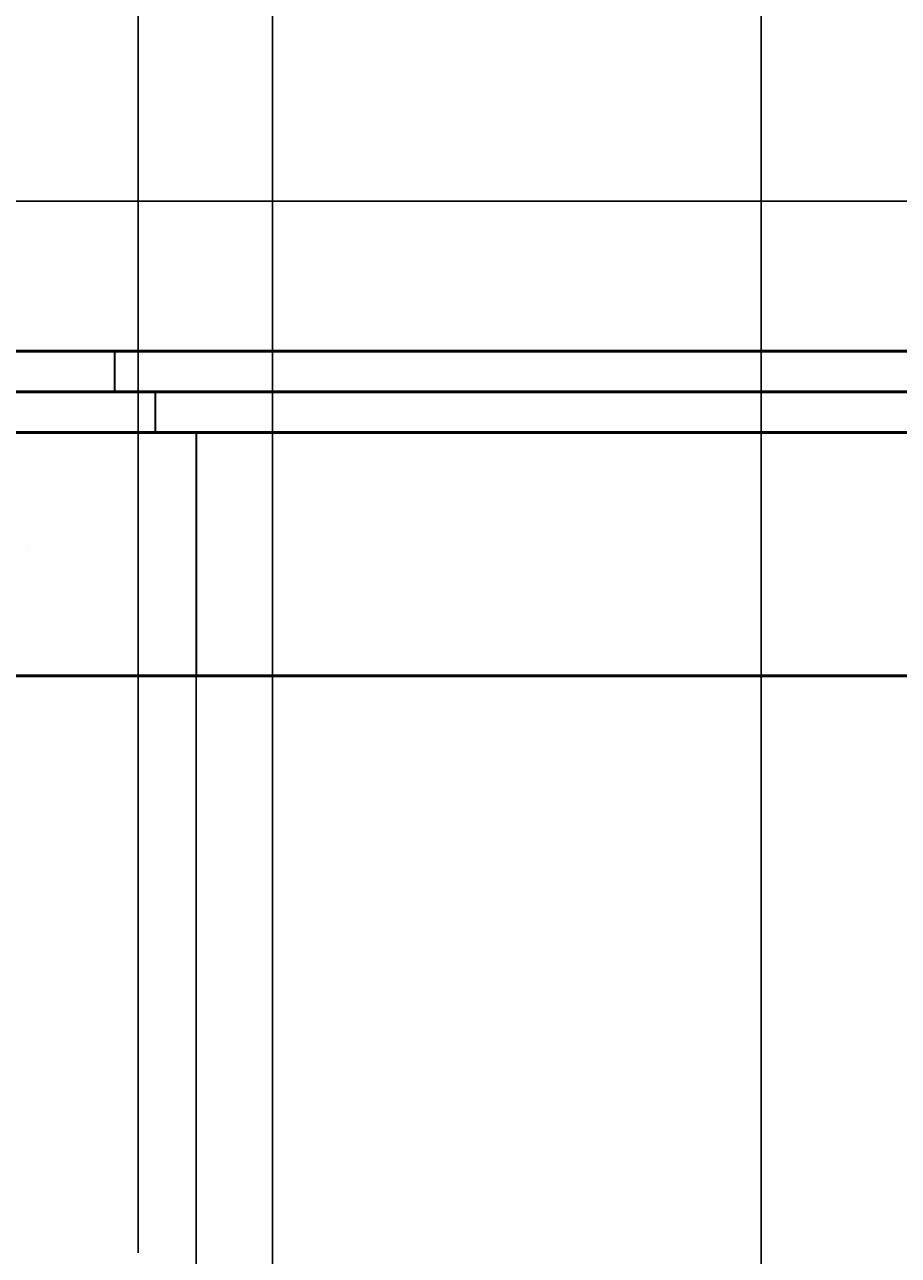
# Model space of a CAD drawing. Units: inches. Extents: x 2812 to 3051, y 1398 to 1659.
# Tile 38 of 65: x 2966 to 2988, y 1468 to 1498. Entities that reach past the tile are written whole.
import ezdxf

# ---------------------------------------------------------------- set-up
doc = ezdxf.new("R2010")
doc.units = ezdxf.units.IN
for name, color, linetype, lineweight in [('A-ANNO-DIMS', 2, 'Continuous', 18), ('S-CONC', 7, 'Continuous', 50), ('S-CONC-PATT', 8, 'Continuous', 18), ('S-CONC-SLAB', 7, 'Continuous', 35)]:
    doc.layers.add(name, color=color, linetype=linetype, lineweight=lineweight)
doc.styles.get("Standard").update_dxf_attribs({"font": 'arial.ttf'})
doc.dimstyles.get("Standard").update_dxf_attribs({"dimtxt": 0.18, "dimasz": 0.18, "dimexe": 0.18, "dimexo": 0.0625, "dimgap": 0.09, "dimtad": 0, "dimtih": 1, "dimtoh": 1, "dimdec": 4, "dimzin": 0, "dimdsep": 46, "dimtxsty": 'Standard', "dimcen": 0.09, "dimadec": 0, "dimazin": 0, "dimtfac": 1, "dimtdec": 4, "dimtofl": 0, "dimtmove": 0, "dimatfit": 3, "dimfxl": 1, "dimtolj": 1, "dimtzin": 0, "dimarcsym": 0})

# ---------------------------------------------------------------- blocks, each defined once
blk = doc.blocks.new('COVER-SLAB-PLAN')
for p, q in [((2, 7), (2, 8)), ((1, 6), (1, 7)), ((1, 7), (2, 7)), ((0, 6), (0, 0)), ((0, 6), (1, 6))]:
    blk.add_line(p, q)
blk = doc.blocks.new('*D31')
at = {"layer": 'A-ANNO-DIMS', "color": 0, "lineweight": -2, "transparency": 16777216}
for p, q in [((2972.272, 1594.192), (2972.272, 1397.505)), ((2961.385, 1559.757), (2961.385, 1397.505)), ((2961.565, 1397.685), (2966.373, 1397.685)), ((2972.092, 1397.685), (2967.283, 1397.685))]:
    blk.add_line(p, q, dxfattribs=at)
at = {"layer": 'A-ANNO-DIMS', "color": 0, "transparency": 16777216}
for points in [[(2961.565, 1397.715), (2961.565, 1397.655), (2961.385, 1397.685)], [(2972.092, 1397.715), (2972.092, 1397.655), (2972.272, 1397.685)]]:
    blk.add_solid(points, dxfattribs=at)
at = {"layer": 'Defpoints', "color": 0, "transparency": 16777216}
for p in [(2972.272, 1594.254), (2961.385, 1559.82), (2972.272, 1397.685)]:
    blk.add_point(p, dxfattribs=at)
at = {"layer": 'A-ANNO-DIMS', "color": 0, "transparency": 16777216, "insert": (2966.828, 1397.685), "char_height": 0.18, "attachment_point": 5}
blk.add_mtext('\\A1;10.887', dxfattribs=at)
blk = doc.blocks.new('*D32')
at = {"layer": 'A-ANNO-DIMS', "color": 0, "lineweight": -2, "transparency": 16777216}
for p, q in [((2984.316, 1598.757), (2984.316, 1397.505)), ((2972.272, 1594.192), (2972.272, 1397.505)), ((2972.452, 1397.685), (2977.839, 1397.685)), ((2984.136, 1397.685), (2978.748, 1397.685))]:
    blk.add_line(p, q, dxfattribs=at)
at = {"layer": 'A-ANNO-DIMS', "color": 0, "transparency": 16777216}
for points in [[(2972.452, 1397.715), (2972.452, 1397.655), (2972.272, 1397.685)], [(2984.136, 1397.715), (2984.136, 1397.655), (2984.316, 1397.685)]]:
    blk.add_solid(points, dxfattribs=at)
at = {"layer": 'Defpoints', "color": 0, "transparency": 16777216}
for p in [(2984.316, 1598.82), (2972.272, 1594.254), (2984.316, 1397.685)]:
    blk.add_point(p, dxfattribs=at)
at = {"layer": 'A-ANNO-DIMS', "color": 0, "transparency": 16777216, "insert": (2978.294, 1397.685), "char_height": 0.18, "attachment_point": 5}
blk.add_mtext('\\A1;12.044', dxfattribs=at)
blk = doc.blocks.new('*D46')
at = {"layer": 'A-ANNO-DIMS', "color": 0, "lineweight": -2, "transparency": 16777216}
for p, q in [((2941.385, 1487.973), (2941.385, 1397.505)), ((2970.385, 1487.973), (2970.385, 1397.505)), ((2941.565, 1397.685), (2955.664, 1397.685)), ((2970.205, 1397.685), (2956.106, 1397.685))]:
    blk.add_line(p, q, dxfattribs=at)
at = {"layer": 'A-ANNO-DIMS', "color": 0, "transparency": 16777216}
for points in [[(2941.565, 1397.715), (2941.565, 1397.655), (2941.385, 1397.685)], [(2970.205, 1397.715), (2970.205, 1397.655), (2970.385, 1397.685)]]:
    blk.add_solid(points, dxfattribs=at)
at = {"layer": 'Defpoints', "color": 0, "transparency": 16777216}
for p in [(2941.385, 1488.035), (2970.385, 1488.035), (2970.385, 1397.685)]:
    blk.add_point(p, dxfattribs=at)
at = {"layer": 'A-ANNO-DIMS', "color": 0, "transparency": 16777216, "insert": (2955.885, 1397.685), "char_height": 0.18, "attachment_point": 5}
blk.add_mtext('\\A1;29', dxfattribs=at)
blk = doc.blocks.new('*D47')
at = {"layer": 'A-ANNO-DIMS', "color": 0, "lineweight": -2, "transparency": 16777216}
for p, q in [((2970.385, 1487.973), (2970.385, 1397.505)), ((3006.385, 1487.973), (3006.385, 1397.505)), ((2970.565, 1397.685), (2988.166, 1397.685)), ((3006.205, 1397.685), (2988.604, 1397.685))]:
    blk.add_line(p, q, dxfattribs=at)
at = {"layer": 'A-ANNO-DIMS', "color": 0, "transparency": 16777216}
for points in [[(2970.565, 1397.715), (2970.565, 1397.655), (2970.385, 1397.685)], [(3006.205, 1397.715), (3006.205, 1397.655), (3006.385, 1397.685)]]:
    blk.add_solid(points, dxfattribs=at)
at = {"layer": 'Defpoints', "color": 0, "transparency": 16777216}
for p in [(2970.385, 1488.035), (3006.385, 1488.035), (3006.385, 1397.685)]:
    blk.add_point(p, dxfattribs=at)
at = {"layer": 'A-ANNO-DIMS', "color": 0, "transparency": 16777216, "insert": (2988.385, 1397.685), "char_height": 0.18, "attachment_point": 5}
blk.add_mtext('\\A1;36', dxfattribs=at)
blk = doc.blocks.new('*D55')
at = {"layer": 'A-ANNO-DIMS', "color": 0, "lineweight": -2, "transparency": 16777216}
for p, q in [((2850.811, 1493.738), (3051.178, 1493.738)), ((3050.998, 1493.558), (3050.998, 1491.069)), ((3050.998, 1488.215), (3050.998, 1490.705)), ((2850.811, 1488.035), (3051.178, 1488.035))]:
    blk.add_line(p, q, dxfattribs=at)
at = {"layer": 'A-ANNO-DIMS', "color": 0, "transparency": 16777216}
for points in [[(3050.968, 1493.558), (3051.028, 1493.558), (3050.998, 1493.738)], [(3050.968, 1488.215), (3051.028, 1488.215), (3050.998, 1488.035)]]:
    blk.add_solid(points, dxfattribs=at)
at = {"layer": 'Defpoints', "color": 0, "transparency": 16777216}
for p in [(2850.748, 1493.738), (3050.998, 1493.738), (2850.748, 1488.035)]:
    blk.add_point(p, dxfattribs=at)
at = {"layer": 'A-ANNO-DIMS', "color": 0, "transparency": 16777216, "insert": (3050.998, 1490.887), "char_height": 0.18, "attachment_point": 5}
blk.add_mtext('\\A1;5.703', dxfattribs=at)
blk = doc.blocks.new('*D69')
at = {"layer": 'A-ANNO-DIMS', "color": 0, "lineweight": -2, "transparency": 16777216}
for p, q in [((2961.385, 1472.098), (2961.385, 1659.35)), ((2968.956, 1467.81), (2968.956, 1659.35)), ((2961.565, 1659.17), (2964.795, 1659.17)), ((2968.776, 1659.17), (2965.546, 1659.17))]:
    blk.add_line(p, q, dxfattribs=at)
at = {"layer": 'A-ANNO-DIMS', "color": 0, "transparency": 16777216}
for points in [[(2961.565, 1659.2), (2961.565, 1659.14), (2961.385, 1659.17)], [(2968.776, 1659.2), (2968.776, 1659.14), (2968.956, 1659.17)]]:
    blk.add_solid(points, dxfattribs=at)
at = {"layer": 'Defpoints', "color": 0, "transparency": 16777216}
for p in [(2968.956, 1659.17), (2961.385, 1472.035), (2968.956, 1467.747)]:
    blk.add_point(p, dxfattribs=at)
at = {"layer": 'A-ANNO-DIMS', "color": 0, "transparency": 16777216, "insert": (2965.17, 1659.17), "char_height": 0.18, "attachment_point": 5}
blk.add_mtext('\\A1;7.571', dxfattribs=at)

msp = doc.modelspace()

# ---------------------------------------------------------------- hatches: boundary and pattern name
at = {"layer": 'S-CONC-PATT'}
h = msp.add_hatch(dxfattribs=at)
h.set_pattern_fill('AR-SAND', color=256, scale=0.3)
h.paths.add_polyline_path([(3036.3849, 1416.0354), (3027.3849, 1416.0354), (2826.3849, 1416.0354), (2826.3849, 1410.0354), (2835.3849, 1410.0354), (3036.3849, 1410.0354)])
h.paths.add_polyline_path([(2970.3849, 1488.0354), (2969.3849, 1488.0354), (2941.3849, 1488.0354), (2941.3849, 1482.0354), (2970.3849, 1482.0354)])
h.paths.add_polyline_path([(3036.3849, 1488.0354), (3035.3849, 1488.0354), (3006.3849, 1488.0354), (3006.3849, 1482.0354), (3027.3849, 1482.0354), (3036.3849, 1482.0354)])
h.paths.add_polyline_path([(3034.3849, 1490.0354), (3008.3849, 1490.0354), (3008.3849, 1489.0354), (3034.3849, 1489.0354)])
h.paths.add_polyline_path([(3035.3849, 1489.0354), (3034.3849, 1489.0354), (3007.3849, 1489.0354), (3007.3849, 1488.0354), (3035.3849, 1488.0354)])
h.paths.add_polyline_path([(2968.3849, 1490.0354), (2943.3849, 1490.0354), (2943.3849, 1489.0354), (2968.3849, 1489.0354)])
h.paths.add_polyline_path([(2969.3849, 1489.0354), (2968.3849, 1489.0354), (2942.3849, 1489.0354), (2942.3849, 1488.0354), (2969.3849, 1488.0354)])
h.paths.add_polyline_path([(2896.3849, 1488.0354), (2826.3849, 1488.0354), (2826.3849, 1482.0354), (2896.3849, 1482.0354)])
h.paths.add_polyline_path([(2895.3849, 1489.0354), (2894.3849, 1489.0354), (2827.3849, 1489.0354), (2827.3849, 1488.0354), (2895.3849, 1488.0354)])
h.paths.add_polyline_path([(2894.3849, 1490.0354), (2828.3849, 1490.0354), (2828.3849, 1489.0354), (2894.3849, 1489.0354)])
h = msp.add_hatch(dxfattribs=at)
h.set_pattern_fill('AR-CONC', color=256, scale=0.3)
h.paths.add_polyline_path([(2896.3849, 1488.0354), (2826.3849, 1488.0354), (2826.3849, 1482.0354), (2896.3849, 1482.0354)])
h.paths.add_polyline_path([(2970.3849, 1488.0354), (2941.3849, 1488.0354), (2941.3849, 1482.0354), (2970.3849, 1482.0354)])
h.paths.add_polyline_path([(2968.3849, 1490.0354), (2943.3849, 1490.0354), (2943.3849, 1489.0354), (2968.3849, 1489.0354)])
h.paths.add_polyline_path([(2969.3849, 1489.0354), (2968.3849, 1489.0354), (2943.3849, 1489.0354), (2942.3849, 1489.0354), (2942.3849, 1488.0354), (2969.3849, 1488.0354)])
h.paths.add_polyline_path([(3036.3849, 1488.0354), (3035.3849, 1488.0354), (3006.3849, 1488.0354), (3006.3849, 1482.0354), (3027.3849, 1482.0354), (3036.3849, 1482.0354)])
h.paths.add_polyline_path([(3035.3849, 1489.0354), (3034.3849, 1489.0354), (3007.3849, 1489.0354), (3007.3849, 1488.0354), (3035.3849, 1488.0354)])
h.paths.add_polyline_path([(3034.3849, 1490.0354), (3008.3849, 1490.0354), (3008.3849, 1489.0354), (3034.3849, 1489.0354)])
h.paths.add_polyline_path([(2895.3849, 1489.0354), (2894.3849, 1489.0354), (2827.3849, 1489.0354), (2827.3849, 1488.0354), (2895.3849, 1488.0354)])
h.paths.add_polyline_path([(2894.3849, 1490.0354), (2828.3849, 1490.0354), (2828.3849, 1489.0354), (2894.3849, 1489.0354)])

# ---------------------------------------------------------------- linework, layer by layer
at = {"layer": 'S-CONC'}
for p, q in [((3034.3849, 1490.0354), (2850.7485, 1490.0354)), ((2850.7485, 1489.0354), (3035.3849, 1489.0354)), ((2850.7485, 1488.0354), (3036.3849, 1488.0354)), ((2850.7485, 1482.0354), (3027.3849, 1482.0354))]:
    msp.add_line(p, q, dxfattribs=at)

# ---------------------------------------------------------------- block references
at = {"layer": 'S-CONC-SLAB', "extrusion": (0, 0, -1), "zscale": -1}
msp.add_blockref('COVER-SLAB-PLAN', (-2970.3848, 1482.035), dxfattribs=at)

# ---------------------------------------------------------------- dimensions: what is measured, and where the dimension line sits
at = {"layer": 'A-ANNO-DIMS'}
for base, p1, p2, override, picture, middle in [((2968.9558, 1659.17), (2961.3849, 1472.0354), (2968.9558, 1467.7474), {"dimdec": 3, "dimlfac": 1, "dimrnd": 0, "dimzin": 0, "dimdsep": 46, "dimlunit": 2}, '*D69', (2965.1704, 1659.17)), ((2984.3156, 1397.6854), (2972.2716, 1594.2541), (2984.3156, 1598.82), {"dimdec": 3, "dimlfac": 1, "dimrnd": 0, "dimzin": 0, "dimdsep": 46, "dimlunit": 2}, '*D32', (2978.2936, 1397.6854)), ((2972.2716, 1397.6854), (2961.3849, 1559.82), (2972.2716, 1594.2541), {"dimdec": 3, "dimlfac": 1, "dimrnd": 0, "dimzin": 0, "dimdsep": 46, "dimlunit": 2}, '*D31', (2966.8282, 1397.6854)), ((2970.3849, 1397.6854), (2941.3849, 1488.0354), (2970.3849, 1488.0354), {"dimdec": 0, "dimlfac": 1, "dimrnd": 0, "dimzin": 0, "dimdsep": 46, "dimlunit": 2}, '*D46', (2955.8849, 1397.6854)), ((3006.3849, 1397.6854), (2970.3849, 1488.0354), (3006.3849, 1488.0354), {"dimdec": 0, "dimlfac": 1, "dimrnd": 0, "dimzin": 0, "dimdsep": 46, "dimlunit": 2}, '*D47', (2988.3849, 1397.6854))]:
    dim = msp.add_linear_dim(base=base, p1=p1, p2=p2, dimstyle='Standard', override=override, dxfattribs=at)
    dim.commit()
    dim.dimension.update_dxf_attribs({"geometry": picture, "text_midpoint": middle})
dim = msp.add_linear_dim(base=(3050.998, 1493.7383), p1=(2850.7485, 1488.0354), p2=(2850.7485, 1493.7383), angle=90, dimstyle='Standard', override={"dimdec": 3, "dimlfac": 1, "dimrnd": 0, "dimzin": 0, "dimdsep": 46, "dimlunit": 2}, dxfattribs=at)
dim.commit()
dim.dimension.update_dxf_attribs({"geometry": '*D55', "text_midpoint": (3050.998, 1490.8868)})

doc.saveas('drawing.dxf')
